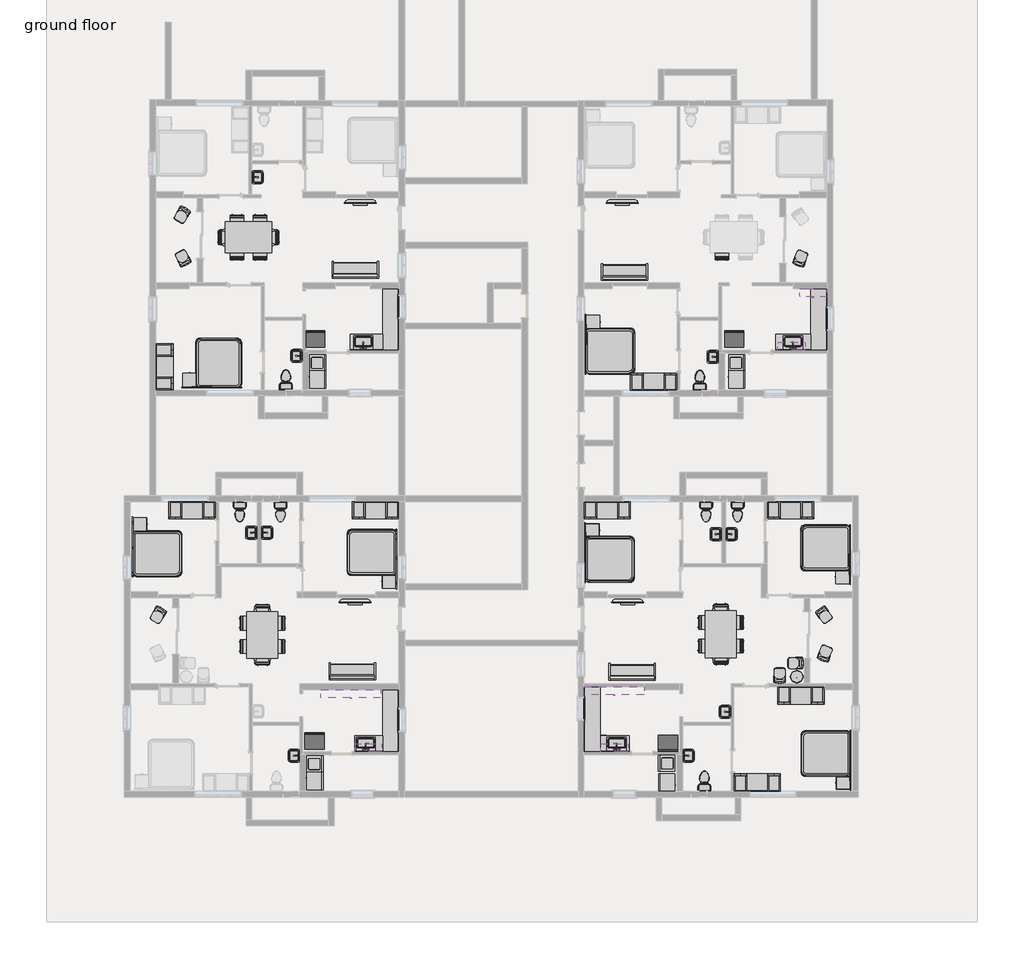
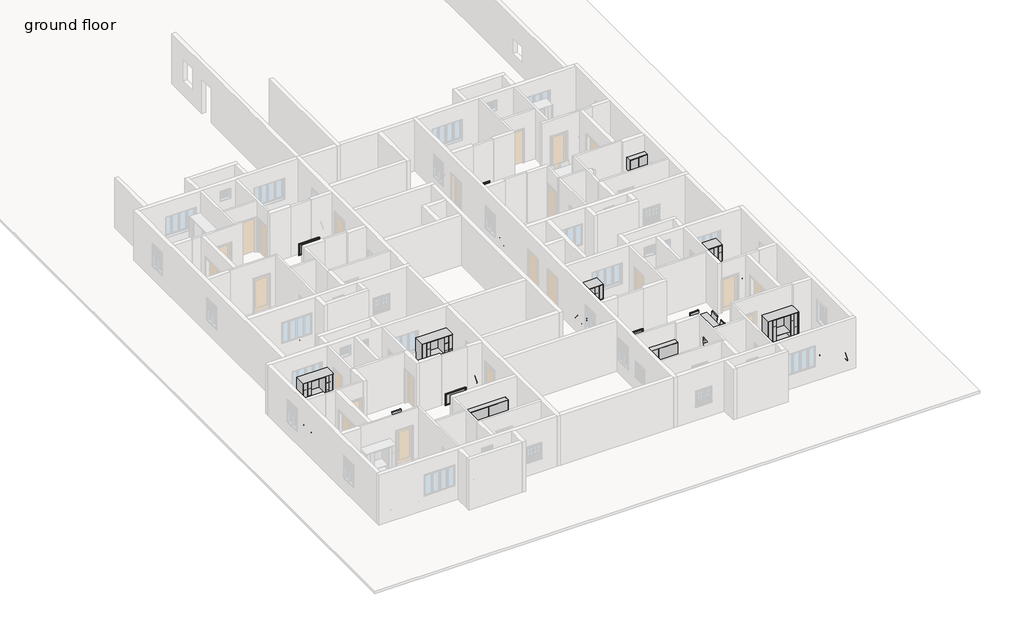
# One storey, part 11 of 16: 80 furniture elements, 21 flow terminals, 12 proxies.
# Revit data of these elements (continued)
# Elements 72, 73, 74 (IfcFurniture, "Counter Top : 24\" Depth")
#   Length = 7' - 11 1/2"
#   Phase Created = New Construction
#   Materials on its faces: "Counter Top"
# Element 75 (IfcFurniture, "Counter Top : 24\" Depth")
#   Length = 8' - 4 1/2"
#   Phase Created = New Construction
#   Materials on its faces: "Counter Top"
# Element 76 (IfcFurniture, "Counter Top w Sink Hole : 24\" Depth")
#   Sink Opening Width = 2' - 3"
#   Sink Opening Depth = 1' - 3"
#   Sink Location To Wall = 0' - 6"
#   Sink Location = 1' - 7.49482"
#   Length = 3' - 9.11988"
#   Phase Created = New Construction
#   Materials on its faces: "Counter Top"
# Element 77 (IfcFurniture, "Counter Top w Sink Hole : 24\" Depth")
#   Sink Opening Width = 2' - 3"
#   Sink Opening Depth = 1' - 3"
#   Sink Location To Wall = 0' - 6"
#   Sink Location = 2' - 2.13425"
#   Length = 3' - 7 1/2"
#   Phase Created = New Construction
#   Materials on its faces: "Counter Top"
# Element 78 (IfcFurniture, "Counter Top w Sink Hole : 24\" Depth")
#   Sink Opening Width = 2' - 3"
#   Sink Opening Depth = 1' - 3"
#   Sink Location To Wall = 0' - 6"
#   Sink Location = 2' - 6.00652"
#   Length = 4' - 2 1/4"
#   Phase Created = New Construction
#   Materials on its faces: "Counter Top"
# Element 79 (IfcFurniture, "Counter Top w Sink Hole : 24\" Depth")
#   Sink Opening Width = 2' - 3"
#   Sink Opening Depth = 1' - 3"
#   Sink Location To Wall = 0' - 6"
#   Sink Location = 2' - 3.62846"
#   Length = 4' - 6"
#   Phase Created = New Construction
#   Materials on its faces: "Counter Top"
# Elements 80, 81, 82, 83, 84, 85, 86, 87 (IfcFurniture, "Entertainment Center : 72\" x 72\" x 24\"")
#   Phase Created = New Construction
#   Materials on its faces: "Steel, Chrome Plated", "Glass - Clear, Grey"
# Elements 88, 89, 90, 91, 92, 93, 94, 95 (IfcFurniture, "Seating-Auditorium : 18\" x 24\" x 30\"")
#   Phase Created = New Construction
#   Materials on its faces: "Steel, Paint Finish, Dark Gray, Matte", "Linen, Beige"
# Elements 96, 97, 98, 99 (IfcFurniture, "Sofa : 72\"")
#   Phase Created = New Construction
#   Materials on its faces: "Cherry", "Linen, Beige"
# Elements 100, 101, 102, 103 (IfcFurniture, "TV - Flat Screen : 50\"")
#   Stand = yes
#   Phase Created = New Construction
#   Materials on its faces: "TV - Black", "TV - Glass", "TV - Screen"
# Elements 104, 105, 106 (IfcFurniture, "Table-Conference2 w Chairs : 48\" x 144\"")
#   Phase Created = New Construction
#   Materials on its faces: "Wood - Cherry"
# Element 107 (IfcFurniture, "Table-Trio End : 20\" Diameter")
#   Phase Created = New Construction
#   Materials on its faces: "Wood - Birch", "Laminate - Ivory,Matte"
# Elements 108, 109, 110, 111 (IfcFurniture, "Upper Cabinet-Double Door-Wall : 42\"")
#   Phase Created = New Construction
#   Materials on its faces: "Cabinets - Handles", "Cabinet"
# Elements 112, 113 (IfcFurniture, "Upper Cabinet-Double Door-Wall : 42\" 3")
#   Phase Created = New Construction
#   Materials on its faces: "Cabinets - Handles", "Cabinet"
# Materials
#   "Metal - Paint Finish - Ivory,Glossy": colour RGB 247 247 239, transparency 0
#   "Metal - Paint Finish - Ivory,Matte": colour RGB 247 247 239, transparency 0
#   "Steel, Polished": class "Metal", colour RGB 192 192 192, transparency 0, Description = "Polished steel", Cost = 0
#   "Porcelain, Linen": class "Ceramic", colour RGB 249 239 230, transparency 0, Description = "Porcelain, linen", Cost = 0
#   "Laminate, Linen, Matte": class "Plastic", colour RGB 249 239 230, transparency 0, Description = "Plastic Laminate - Linen, Matte", Cost = 0
#   "Cabinets": colour RGB 249 249 249, transparency 0
#   "Cabinets - Handles": colour RGB 57 57 57, transparency 0
#   "Plastic - Black": colour RGB 0 0 0, transparency 0.7
#   "Textile - Slate Blue": colour RGB 98 102 118, transparency 0
#   "Linen, Beige": class "Textile", colour RGB 249 239 230, transparency 0, Description = "Linen, beige", Cost = 0
#   "Steel, Paint Finish, Dark Gray, Matte": class "Metal", colour RGB 0 0 0, transparency 0, Description = "Steel, paint finish, dark gray, matte", Cost = 0
#   "Cherry": class "Wood", colour RGB 226 177 128, transparency 0, Description = "Prunus Serotina", Cost = 0
#   "Wood - Cherry": colour RGB 151 75 0, transparency 0
#   "Wood - Birch": colour RGB 230 196 162, transparency 0
#   "Laminate - Ivory,Matte": colour RGB 127 127 127, transparency 0
#   "Metal - Chrome": colour RGB 57 57 57, transparency 0
#   "wood 2": class "Wood", colour RGB 196 146 67, transparency 0
#   "ss": class "Metal", colour RGB 189 187 185, transparency 0
#   "new wood": class "Wood", colour RGB 133 62 31, transparency 0
#   "fabric 2": class "Fabric", colour RGB 198 193 133, transparency 0
#   "wood light": class "Wood", colour RGB 198 165 122, transparency 0
#   "fabric": class "Fabric", colour RGB 198 193 133, transparency 0
#   "Cabinet": colour RGB 204 122 2, transparency 0
#   "Counter Top": class "Wood", colour RGB 226 177 128, transparency 0
#   "Steel, Chrome Plated": class "Metal", colour RGB 17 17 17, transparency 0, Description = "Chromiuim plated steel", Cost = 0
#   "Glass - Clear, Grey": class "Glass", colour RGB 252 255 255, transparency 0.64
#   "TV - Black": colour RGB 49 49 49, transparency 0
#   "TV - Glass": colour RGB 157 157 157, transparency 0.9
#   "TV - Screen": colour RGB 0 0 0, transparency 0
